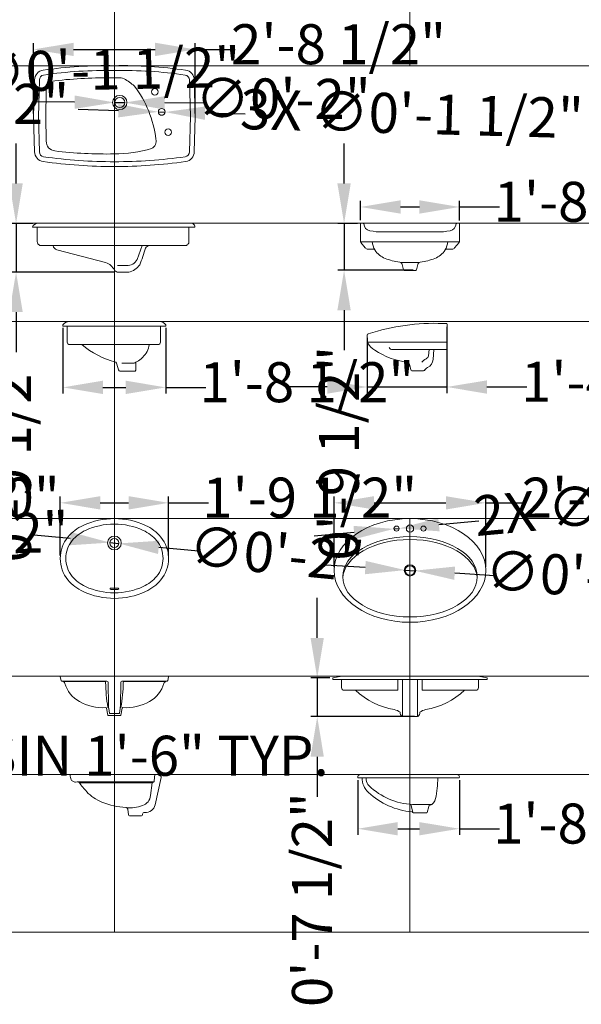
# Model space of a CAD drawing. Units: inches. Extents: x 2138 to 3265, y 2149 to 3392.
# Tile 8 of 13: x 2928 to 3040, y 3051 to 3248. Entities that reach past the tile are written whole.
import ezdxf

# ---------------------------------------------------------------- set-up
doc = ezdxf.new("R2010")
doc.units = ezdxf.units.IN
for name, color, linetype, lineweight in [('A-ANNO-DIMS', 2, 'Continuous', 18), ('A-DETL-GRID', 1, 'Continuous', 13), ('Washbasin-detail', 251, 'Continuous', 13), ('Washbasin-outline', 250, 'Continuous', 20)]:
    doc.layers.add(name, color=color, linetype=linetype, lineweight=lineweight)
doc.styles.get("Standard").update_dxf_attribs({"font": 'arial.ttf'})
doc.dimstyles.new('ISO-25', dxfattribs={"dimtxt": 8, "dimasz": 8, "dimexe": 1.25, "dimexo": 0.625, "dimtad": 0, "dimdec": 1, "dimlunit": 4, "dimtxsty": 'Standard', "dimcen": 2.5, "dimadec": 0, "dimazin": 0, "dimtfac": 1, "dimtdec": 1, "dimtmove": 0, "dimatfit": 3, "dimfxl": 1, "dimarcsym": 0})

# ---------------------------------------------------------------- blocks, each defined once
blk = doc.blocks.new('BASIN-WALLHUNG-SIDE')
for p, q in [((16.94, 8.23), (16.8, 6.96)), ((0.38, 6.97), (0.83, 6.75)), ((1.41, 6.77), (1.08, 6.71)), ((1.41, 6.77), (16.72, 6.77)), ((1.8, 6.61), (16.41, 6.61)), ((16.36, 6.61), (16.07, 4.02)), ((11.67, 0.17), (11.54, 1.3)), ((14.45, 0.17), (14.46, 0.29)), ((11.87, 0), (14.25, 0))]:
    blk.add_line(p, q)
for points in [[(17.61, 8.23), (0.08, 8.23, 0.427055), (0, 8.15, 0.060898), (0.18, 7.2)], [(17.81, 8.05), (18.01, 7.98, -0.38584), (18.2, 7.66), (16.99, 2.18)]]:
    blk.add_lwpolyline(points, format="xyb")
for centre, radius, start, end in [((17.61, 8.11), 0.119, 11.3189, 90), ((17.85, 8.16), 0.119, 191.3189, 251.9239), ((0.56, 7.33), 0.396, 197.6362, 243.4349), ((1.01, 7.1), 0.396, 243.4349, 279.8522), ((1.48, 6.38), 0.396, 36.3193, 99.8522), ((18.06, 18.57), 20.18, 216.3193, 223.028), ((16.41, 7.01), 0.396, 270, 353.6234), ((9.38, 10.47), 8.31, 223.028, 248.5761), ((13.71, 4.28), 2.37, 288.7646, 353.6234), ((12.27, 17.83), 16.23, 248.5761, 266.122), ((12.12, 7.8), 6.22, 261.2493, 292.2117), ((15.05, 2.61), 1.98, 265.1357, 347.5295), ((11.15, 1.25), 0.396, 6.7098, 86.122), ((11.87, 0.2), 0.198, 186.7098, 270), ((14.25, 0.2), 0.198, 270, 353.2902), ((14.85, 0.25), 0.396, 85.1357, 173.2902)]:
    blk.add_arc(centre, radius, start, end)
blk = doc.blocks.new('*D49')
at = {"layer": 'A-ANNO-DIMS', "color": 0, "lineweight": -2, "transparency": 16777216}
for p, q in [((2878.67, 3097.91), (2878.67, 3101.27)), ((2896.9, 3097.91), (2896.9, 3101.27)), ((2886.67, 3100.02), (2888.9, 3100.02)), ((2896.9, 3100.02), (2904.9, 3100.02))]:
    blk.add_line(p, q, dxfattribs=at)
at = {"layer": 'A-ANNO-DIMS', "color": 0, "transparency": 16777216}
for points in [[(2886.67, 3101.35), (2886.67, 3098.69), (2878.67, 3100.02)], [(2888.9, 3101.35), (2888.9, 3098.69), (2896.9, 3100.02)]]:
    blk.add_solid(points, dxfattribs=at)
at = {"layer": 'Defpoints', "color": 0, "transparency": 16777216}
for p in [(2896.9, 3100.02), (2878.67, 3097.29), (2896.9, 3097.29)]:
    blk.add_point(p, dxfattribs=at)
at = {"layer": 'A-ANNO-DIMS', "color": 0, "transparency": 16777216, "insert": (2948.05, 3100.02), "char_height": 8, "attachment_point": 5}
blk.add_mtext('BASIN 1\'-6" TYP.', dxfattribs=at)
blk = doc.blocks.new('*D82')
at = {"layer": 'A-ANNO-DIMS', "color": 0, "lineweight": -2, "transparency": 16777216}
for p, q in [((2930.43, 3229.45), (2930.43, 3243.52)), ((2938.43, 3242.27), (2954.71, 3242.27)), ((2962.71, 3229.45), (2962.71, 3243.52)), ((2962.71, 3242.27), (2970.71, 3242.27))]:
    blk.add_line(p, q, dxfattribs=at)
at = {"layer": 'A-ANNO-DIMS', "color": 0, "transparency": 16777216}
for points in [[(2938.43, 3243.6), (2938.43, 3240.94), (2930.43, 3242.27)], [(2954.71, 3243.6), (2954.71, 3240.94), (2962.71, 3242.27)]]:
    blk.add_solid(points, dxfattribs=at)
at = {"layer": 'Defpoints', "color": 0, "transparency": 16777216}
for p in [(2962.71, 3242.27), (2930.43, 3228.82), (2962.71, 3228.82)]:
    blk.add_point(p, dxfattribs=at)
at = {"layer": 'A-ANNO-DIMS', "color": 0, "transparency": 16777216, "insert": (2991.36, 3242.27), "char_height": 8, "attachment_point": 5}
blk.add_mtext('2\'-8 1/2"', dxfattribs=at)
blk = doc.blocks.new('*D83')
at = {"layer": 'A-ANNO-DIMS', "color": 0, "lineweight": -2, "transparency": 16777216}
for p, q in [((2926.93, 3215.47), (2926.93, 3223.47)), ((2930.28, 3207.47), (2925.68, 3207.47)), ((2926.93, 3207.47), (2926.93, 3197.76)), ((2946.5, 3197.76), (2925.68, 3197.76)), ((2926.93, 3189.76), (2926.93, 3181.76))]:
    blk.add_line(p, q, dxfattribs=at)
at = {"layer": 'A-ANNO-DIMS', "color": 0, "transparency": 16777216}
for points in [[(2925.59, 3215.47), (2928.26, 3215.47), (2926.93, 3207.47)], [(2925.59, 3189.76), (2928.26, 3189.76), (2926.93, 3197.76)]]:
    blk.add_solid(points, dxfattribs=at)
at = {"layer": 'Defpoints', "color": 0, "transparency": 16777216}
for p in [(2930.91, 3207.47), (2926.93, 3197.76), (2947.13, 3197.76)]:
    blk.add_point(p, dxfattribs=at)
at = {"layer": 'A-ANNO-DIMS', "color": 0, "transparency": 16777216, "insert": (2926.93, 3161.18), "char_height": 8, "attachment_point": 5, "rotation": 90}
blk.add_mtext('0\'-9 1/2"', dxfattribs=at)
blk = doc.blocks.new('*D84')
at = {"layer": 'A-ANNO-DIMS', "color": 0, "lineweight": -2, "transparency": 16777216}
for p, q in [((2936.28, 3186.58), (2936.28, 3173.45)), ((2956.83, 3186.58), (2956.83, 3173.45)), ((2944.28, 3174.7), (2948.83, 3174.7)), ((2956.83, 3174.7), (2964.83, 3174.7))]:
    blk.add_line(p, q, dxfattribs=at)
at = {"layer": 'A-ANNO-DIMS', "color": 0, "transparency": 16777216}
for points in [[(2944.28, 3176.04), (2944.28, 3173.37), (2936.28, 3174.7)], [(2948.83, 3176.04), (2948.83, 3173.37), (2956.83, 3174.7)]]:
    blk.add_solid(points, dxfattribs=at)
at = {"layer": 'Defpoints', "color": 0, "transparency": 16777216}
for p in [(2936.28, 3187.21), (2956.83, 3187.21), (2956.83, 3174.7)]:
    blk.add_point(p, dxfattribs=at)
at = {"layer": 'A-ANNO-DIMS', "color": 0, "transparency": 16777216, "insert": (2985.03, 3174.7), "char_height": 8, "attachment_point": 5}
blk.add_mtext('1\'-8 1/2"', dxfattribs=at)
blk = doc.blocks.new('*D85')
at = {"layer": 'A-ANNO-DIMS', "color": 0, "lineweight": -2, "transparency": 16777216}
for p, q in [((2995.75, 3208.1), (2995.75, 3212.02)), ((3003.75, 3210.77), (3007.52, 3210.77)), ((3015.52, 3208.08), (3015.52, 3212.02)), ((3015.52, 3210.77), (3023.52, 3210.77))]:
    blk.add_line(p, q, dxfattribs=at)
at = {"layer": 'A-ANNO-DIMS', "color": 0, "transparency": 16777216}
for points in [[(3003.75, 3212.11), (3003.75, 3209.44), (2995.75, 3210.77)], [(3007.52, 3212.11), (3007.52, 3209.44), (3015.52, 3210.77)]]:
    blk.add_solid(points, dxfattribs=at)
at = {"layer": 'Defpoints', "color": 0, "transparency": 16777216}
for p in [(3015.52, 3210.77), (2995.75, 3207.48), (3015.52, 3207.45)]:
    blk.add_point(p, dxfattribs=at)
at = {"layer": 'A-ANNO-DIMS', "color": 0, "transparency": 16777216, "insert": (3034.4, 3210.77), "char_height": 8, "attachment_point": 5}
blk.add_mtext('1\'-8"', dxfattribs=at)
blk = doc.blocks.new('*D86')
at = {"layer": 'A-ANNO-DIMS', "color": 0, "lineweight": -2, "transparency": 16777216}
for p, q in [((2992.46, 3215.48), (2992.46, 3223.48)), ((2995.13, 3207.48), (2991.21, 3207.48)), ((2992.46, 3207.48), (2992.46, 3198.12)), ((3006.25, 3198.12), (2991.21, 3198.12)), ((2992.46, 3190.12), (2992.46, 3182.12))]:
    blk.add_line(p, q, dxfattribs=at)
at = {"layer": 'A-ANNO-DIMS', "color": 0, "transparency": 16777216}
for points in [[(2991.12, 3215.48), (2993.79, 3215.48), (2992.46, 3207.48)], [(2991.12, 3190.12), (2993.79, 3190.12), (2992.46, 3198.12)]]:
    blk.add_solid(points, dxfattribs=at)
at = {"layer": 'Defpoints', "color": 0, "transparency": 16777216}
for p in [(2995.75, 3207.48), (2992.46, 3198.12), (3006.88, 3198.12)]:
    blk.add_point(p, dxfattribs=at)
at = {"layer": 'A-ANNO-DIMS', "color": 0, "transparency": 16777216, "insert": (2992.46, 3161.54), "char_height": 8, "attachment_point": 5, "rotation": 90}
blk.add_mtext('0\'-9 1/2"', dxfattribs=at)
blk = doc.blocks.new('*D87')
at = {"layer": 'A-ANNO-DIMS', "color": 0, "lineweight": -2, "transparency": 16777216}
for p, q in [((3012.99, 3186.82), (3012.99, 3173.53)), ((2997.1, 3184.61), (2997.1, 3173.53)), ((2989.1, 3174.78), (2981.1, 3174.78)), ((2997.1, 3174.78), (3012.99, 3174.78)), ((3020.99, 3174.78), (3028.99, 3174.78))]:
    blk.add_line(p, q, dxfattribs=at)
at = {"layer": 'A-ANNO-DIMS', "color": 0, "transparency": 16777216}
for points in [[(2989.1, 3176.11), (2989.1, 3173.44), (2997.1, 3174.78)], [(3020.99, 3176.11), (3020.99, 3173.44), (3012.99, 3174.78)]]:
    blk.add_solid(points, dxfattribs=at)
at = {"layer": 'Defpoints', "color": 0, "transparency": 16777216}
for p in [(3012.99, 3187.44), (2997.1, 3185.23), (3012.99, 3174.78)]:
    blk.add_point(p, dxfattribs=at)
at = {"layer": 'A-ANNO-DIMS', "color": 0, "transparency": 16777216, "insert": (3039.87, 3174.78), "char_height": 8, "attachment_point": 5}
blk.add_mtext('1\'-4"', dxfattribs=at)
blk = doc.blocks.new('*D89')
at = {"layer": 'A-ANNO-DIMS', "color": 0, "lineweight": -2, "transparency": 16777216}
for p, q in [((3048.17, 3215.38), (3048.17, 3223.38)), ((3050.93, 3207.38), (3046.92, 3207.38)), ((3048.17, 3207.38), (3048.17, 3199.85)), ((3065.38, 3199.85), (3046.92, 3199.85)), ((3048.17, 3191.85), (3048.17, 3183.85))]:
    blk.add_line(p, q, dxfattribs=at)
at = {"layer": 'A-ANNO-DIMS', "color": 0, "transparency": 16777216}
for points in [[(3046.84, 3215.38), (3049.5, 3215.38), (3048.17, 3207.38)], [(3046.84, 3191.85), (3049.5, 3191.85), (3048.17, 3199.85)]]:
    blk.add_solid(points, dxfattribs=at)
at = {"layer": 'Defpoints', "color": 0, "transparency": 16777216}
for p in [(3051.56, 3207.38), (3048.17, 3199.85), (3066, 3199.85)]:
    blk.add_point(p, dxfattribs=at)
at = {"layer": 'A-ANNO-DIMS', "color": 0, "transparency": 16777216, "insert": (3048.17, 3163.27), "char_height": 8, "attachment_point": 5, "rotation": 90}
blk.add_mtext('0\'-7 1/2"', dxfattribs=at)
blk = doc.blocks.new('*D97')
at = {"layer": 'A-ANNO-DIMS', "color": 0, "lineweight": -2, "transparency": 16777216}
for p, q in [((2876.44, 3139.39), (2876.44, 3152.87)), ((2898.59, 3139.39), (2898.59, 3152.87)), ((2884.44, 3151.62), (2890.59, 3151.62)), ((2898.59, 3151.62), (2906.59, 3151.62))]:
    blk.add_line(p, q, dxfattribs=at)
at = {"layer": 'A-ANNO-DIMS', "color": 0, "transparency": 16777216}
for points in [[(2884.44, 3152.95), (2884.44, 3150.28), (2876.44, 3151.62)], [(2890.59, 3152.95), (2890.59, 3150.28), (2898.59, 3151.62)]]:
    blk.add_solid(points, dxfattribs=at)
at = {"layer": 'Defpoints', "color": 0, "transparency": 16777216}
for p in [(2898.59, 3151.62), (2876.44, 3138.77), (2898.59, 3138.77)]:
    blk.add_point(p, dxfattribs=at)
at = {"layer": 'A-ANNO-DIMS', "color": 0, "transparency": 16777216, "insert": (2920.58, 3151.62), "char_height": 8, "attachment_point": 5}
blk.add_mtext('1\'-10"', dxfattribs=at)
blk = doc.blocks.new('*D98')
at = {"layer": 'A-ANNO-DIMS', "color": 0, "lineweight": -2, "transparency": 16777216}
for p, q in [((2935.75, 3141.12), (2935.75, 3152.87)), ((2957.4, 3141.12), (2957.4, 3152.87)), ((2943.75, 3151.62), (2949.4, 3151.62)), ((2957.4, 3151.62), (2965.4, 3151.62))]:
    blk.add_line(p, q, dxfattribs=at)
at = {"layer": 'A-ANNO-DIMS', "color": 0, "transparency": 16777216}
for points in [[(2943.75, 3152.95), (2943.75, 3150.28), (2935.75, 3151.62)], [(2949.4, 3152.95), (2949.4, 3150.28), (2957.4, 3151.62)]]:
    blk.add_solid(points, dxfattribs=at)
at = {"layer": 'Defpoints', "color": 0, "transparency": 16777216}
for p in [(2957.4, 3151.62), (2935.75, 3140.5), (2957.4, 3140.5)]:
    blk.add_point(p, dxfattribs=at)
at = {"layer": 'A-ANNO-DIMS', "color": 0, "transparency": 16777216, "insert": (2985.6, 3151.62), "char_height": 8, "attachment_point": 5}
blk.add_mtext('1\'-9 1/2"', dxfattribs=at)
blk = doc.blocks.new('*D99')
at = {"layer": 'A-ANNO-DIMS', "color": 0, "lineweight": -2, "transparency": 16777216}
for p, q in [((2990.46, 3138.73), (2990.46, 3152.87)), ((3020.79, 3138.73), (3020.79, 3152.87)), ((2998.46, 3151.62), (3012.79, 3151.62)), ((3020.79, 3151.62), (3028.79, 3151.62))]:
    blk.add_line(p, q, dxfattribs=at)
at = {"layer": 'A-ANNO-DIMS', "color": 0, "transparency": 16777216}
for points in [[(2998.46, 3152.95), (2998.46, 3150.28), (2990.46, 3151.62)], [(3012.79, 3152.95), (3012.79, 3150.28), (3020.79, 3151.62)]]:
    blk.add_solid(points, dxfattribs=at)
at = {"layer": 'Defpoints', "color": 0, "transparency": 16777216}
for p in [(3020.79, 3151.62), (2990.46, 3138.1), (3020.79, 3138.1)]:
    blk.add_point(p, dxfattribs=at)
at = {"layer": 'A-ANNO-DIMS', "color": 0, "transparency": 16777216, "insert": (3049.44, 3151.62), "char_height": 8, "attachment_point": 5}
blk.add_mtext('2\'-6 1/2"', dxfattribs=at)
blk = doc.blocks.new('*D100')
at = {"layer": 'A-ANNO-DIMS', "color": 0, "lineweight": -2, "transparency": 16777216}
for p, q in [((2987.09, 3124.6), (2987.09, 3132.6)), ((2989.61, 3116.6), (2985.84, 3116.6)), ((2987.09, 3116.6), (2987.09, 3108.87)), ((3006.53, 3108.87), (2985.84, 3108.87)), ((2987.09, 3100.87), (2987.09, 3092.87))]:
    blk.add_line(p, q, dxfattribs=at)
at = {"layer": 'A-ANNO-DIMS', "color": 0, "transparency": 16777216}
for points in [[(2985.76, 3124.6), (2988.42, 3124.6), (2987.09, 3116.6)], [(2985.76, 3100.87), (2988.42, 3100.87), (2987.09, 3108.87)]]:
    blk.add_solid(points, dxfattribs=at)
at = {"layer": 'Defpoints', "color": 0, "transparency": 16777216}
for p in [(2990.24, 3116.6), (2987.09, 3108.87), (3007.15, 3108.87)]:
    blk.add_point(p, dxfattribs=at)
at = {"layer": 'A-ANNO-DIMS', "color": 0, "transparency": 16777216, "insert": (2987.09, 3072.29), "char_height": 8, "attachment_point": 5, "rotation": 90}
blk.add_mtext('0\'-7 1/2"', dxfattribs=at)
blk = doc.blocks.new('*D101')
at = {"layer": 'A-ANNO-DIMS', "color": 0, "lineweight": -2, "transparency": 16777216}
for p, q in [((2995.19, 3096.14), (2995.19, 3085.21)), ((3015.5, 3096.19), (3015.5, 3085.21)), ((3003.19, 3086.46), (3007.5, 3086.46)), ((3015.5, 3086.46), (3023.5, 3086.46))]:
    blk.add_line(p, q, dxfattribs=at)
at = {"layer": 'A-ANNO-DIMS', "color": 0, "transparency": 16777216}
for points in [[(3003.19, 3087.79), (3003.19, 3085.13), (2995.19, 3086.46)], [(3007.5, 3087.79), (3007.5, 3085.13), (3015.5, 3086.46)]]:
    blk.add_solid(points, dxfattribs=at)
at = {"layer": 'Defpoints', "color": 0, "transparency": 16777216}
for p in [(2995.19, 3096.77), (3015.5, 3096.81), (3015.5, 3086.46)]:
    blk.add_point(p, dxfattribs=at)
at = {"layer": 'A-ANNO-DIMS', "color": 0, "transparency": 16777216, "insert": (3043.7, 3086.46), "char_height": 8, "attachment_point": 5}
blk.add_mtext('1\'-8 1/2"', dxfattribs=at)
blk = doc.blocks.new('*D121')
at = {"layer": 'A-ANNO-DIMS', "color": 0, "lineweight": -2, "transparency": 16777216}
for p, q in [((2904.18, 3236.4), (2896.19, 3236.24)), ((2878.85, 3235.89), (2870.85, 3235.74)), ((2886.85, 3236.05), (2888.19, 3236.08))]:
    blk.add_line(p, q, dxfattribs=at)
at = {"layer": 'A-ANNO-DIMS', "color": 0, "transparency": 16777216}
for points in [[(2878.82, 3237.23), (2878.88, 3234.56), (2886.85, 3236.05)], [(2896.16, 3237.57), (2896.21, 3234.91), (2888.19, 3236.08)]]:
    blk.add_solid(points, dxfattribs=at)
at = {"layer": 'Defpoints', "color": 0, "transparency": 16777216}
for p in [(2886.85, 3236.05), (2888.19, 3236.08)]:
    blk.add_point(p, dxfattribs=at)
at = {"layer": 'A-ANNO-DIMS', "color": 0, "transparency": 16777216, "insert": (2937.49, 3237.06), "char_height": 8, "attachment_point": 5, "rotation": 1.1379}
blk.add_mtext('3X ∅0\'-1 1/2"', dxfattribs=at)
blk = doc.blocks.new('*D122')
at = {"layer": 'A-ANNO-DIMS', "color": 0, "lineweight": -2, "transparency": 16777216}
for p, q in [((2878.63, 3230.6), (2870.63, 3230.64)), ((2886.63, 3230.56), (2888.4, 3230.55)), ((2904.4, 3230.47), (2896.4, 3230.51))]:
    blk.add_line(p, q, dxfattribs=at)
at = {"layer": 'A-ANNO-DIMS', "color": 0, "transparency": 16777216}
for points in [[(2878.64, 3231.93), (2878.63, 3229.27), (2886.63, 3230.56)], [(2896.41, 3231.84), (2896.4, 3229.18), (2888.4, 3230.55)]]:
    blk.add_solid(points, dxfattribs=at)
at = {"layer": 'Defpoints', "color": 0, "transparency": 16777216}
for p in [(2886.63, 3230.56), (2888.4, 3230.55)]:
    blk.add_point(p, dxfattribs=at)
at = {"layer": 'A-ANNO-DIMS', "color": 0, "transparency": 16777216, "insert": (2920.01, 3230.39), "char_height": 8, "attachment_point": 5, "rotation": 359.7153}
blk.add_mtext('∅0\'-2"', dxfattribs=at)
blk = doc.blocks.new('*D123')
at = {"layer": 'A-ANNO-DIMS', "color": 0, "lineweight": -2, "transparency": 16777216}
for p, q in [((2947.36, 3230.01), (2939.36, 3230.23)), ((2955.35, 3229.79), (2956.69, 3229.75)), ((2972.68, 3229.31), (2964.69, 3229.53))]:
    blk.add_line(p, q, dxfattribs=at)
at = {"layer": 'A-ANNO-DIMS', "color": 0, "transparency": 16777216}
for points in [[(2947.39, 3231.34), (2947.32, 3228.67), (2955.35, 3229.79)], [(2964.72, 3230.86), (2964.65, 3228.19), (2956.69, 3229.75)]]:
    blk.add_solid(points, dxfattribs=at)
at = {"layer": 'Defpoints', "color": 0, "transparency": 16777216}
for p in [(2955.35, 3229.79), (2956.69, 3229.75)]:
    blk.add_point(p, dxfattribs=at)
at = {"layer": 'A-ANNO-DIMS', "color": 0, "transparency": 16777216, "insert": (3005.98, 3228.39), "char_height": 8, "attachment_point": 5, "rotation": 358.4162}
blk.add_mtext('3X ∅0\'-1 1/2"', dxfattribs=at)
blk = doc.blocks.new('*D124')
at = {"layer": 'A-ANNO-DIMS', "color": 0, "lineweight": -2, "transparency": 16777216}
for p, q in [((2938.63, 3231.73), (2930.63, 3231.79)), ((2946.63, 3231.66), (2948.64, 3231.65)), ((2964.64, 3231.52), (2956.64, 3231.59))]:
    blk.add_line(p, q, dxfattribs=at)
at = {"layer": 'A-ANNO-DIMS', "color": 0, "transparency": 16777216}
for points in [[(2938.64, 3233.06), (2938.62, 3230.39), (2946.63, 3231.66)], [(2956.65, 3232.92), (2956.63, 3230.25), (2948.64, 3231.65)]]:
    blk.add_solid(points, dxfattribs=at)
at = {"layer": 'Defpoints', "color": 0, "transparency": 16777216}
for p in [(2946.63, 3231.66), (2948.64, 3231.65)]:
    blk.add_point(p, dxfattribs=at)
at = {"layer": 'A-ANNO-DIMS', "color": 0, "transparency": 16777216, "insert": (2980.25, 3231.4), "char_height": 8, "attachment_point": 5, "rotation": 359.5528}
blk.add_mtext('∅0\'-2"', dxfattribs=at)
blk = doc.blocks.new('*D130')
at = {"layer": 'A-ANNO-DIMS', "color": 0, "lineweight": -2, "transparency": 16777216}
for p, q in [((2904.4, 3143.83), (2896.4, 3143.59)), ((2878.63, 3143.06), (2870.63, 3142.82)), ((2886.63, 3143.3), (2888.41, 3143.35))]:
    blk.add_line(p, q, dxfattribs=at)
at = {"layer": 'A-ANNO-DIMS', "color": 0, "transparency": 16777216}
for points in [[(2878.59, 3144.39), (2878.67, 3141.72), (2886.63, 3143.3)], [(2896.36, 3144.92), (2896.44, 3142.26), (2888.41, 3143.35)]]:
    blk.add_solid(points, dxfattribs=at)
at = {"layer": 'Defpoints', "color": 0, "transparency": 16777216}
for p in [(2886.63, 3143.3), (2888.41, 3143.35)]:
    blk.add_point(p, dxfattribs=at)
at = {"layer": 'A-ANNO-DIMS', "color": 0, "transparency": 16777216, "insert": (2920, 3144.3), "char_height": 8, "attachment_point": 5, "rotation": 1.7228}
blk.add_mtext('∅0\'-2"', dxfattribs=at)
blk = doc.blocks.new('*D131')
at = {"layer": 'A-ANNO-DIMS', "color": 0, "lineweight": -2, "transparency": 16777216}
for p, q in [((2937.73, 3144.46), (2929.77, 3145.24)), ((2945.69, 3143.67), (2947.45, 3143.5)), ((2963.38, 3141.93), (2955.42, 3142.72))]:
    blk.add_line(p, q, dxfattribs=at)
at = {"layer": 'A-ANNO-DIMS', "color": 0, "transparency": 16777216}
for points in [[(2937.86, 3145.78), (2937.6, 3143.13), (2945.69, 3143.67)], [(2955.55, 3144.04), (2955.29, 3141.39), (2947.45, 3143.5)]]:
    blk.add_solid(points, dxfattribs=at)
at = {"layer": 'Defpoints', "color": 0, "transparency": 16777216}
for p in [(2945.69, 3143.67), (2947.45, 3143.5)]:
    blk.add_point(p, dxfattribs=at)
at = {"layer": 'A-ANNO-DIMS', "color": 0, "transparency": 16777216, "insert": (2978.91, 3140.41), "char_height": 8, "attachment_point": 5, "rotation": 354.3826}
blk.add_mtext('∅0\'-2"', dxfattribs=at)
blk = doc.blocks.new('*D132')
at = {"layer": 'A-ANNO-DIMS', "color": 0, "lineweight": -2, "transparency": 16777216}
for p, q in [((3019.38, 3147.98), (3011.42, 3147.24)), ((3002.43, 3146.42), (3003.45, 3146.51)), ((2994.46, 3145.69), (2986.49, 3144.95))]:
    blk.add_line(p, q, dxfattribs=at)
at = {"layer": 'A-ANNO-DIMS', "color": 0, "transparency": 16777216}
for points in [[(3011.29, 3148.57), (3011.54, 3145.92), (3003.45, 3146.51)], [(2994.34, 3147.01), (2994.58, 3144.36), (3002.43, 3146.42)]]:
    blk.add_solid(points, dxfattribs=at)
at = {"layer": 'Defpoints', "color": 0, "transparency": 16777216}
for p in [(3002.43, 3146.42), (3003.45, 3146.51)]:
    blk.add_point(p, dxfattribs=at)
at = {"layer": 'A-ANNO-DIMS', "color": 0, "transparency": 16777216, "insert": (3043.34, 3150.18), "char_height": 8, "attachment_point": 5, "rotation": 5.2513}
blk.add_mtext('2X ∅0\'-1"', dxfattribs=at)
blk = doc.blocks.new('*D133')
at = {"layer": 'A-ANNO-DIMS', "color": 0, "lineweight": -2, "transparency": 16777216}
for p, q in [((2996.7, 3138.67), (2988.72, 3139.17)), ((3004.68, 3138.17), (3006.57, 3138.05)), ((3022.54, 3137.05), (3014.56, 3137.55))]:
    blk.add_line(p, q, dxfattribs=at)
at = {"layer": 'A-ANNO-DIMS', "color": 0, "transparency": 16777216}
for points in [[(2996.78, 3140), (2996.62, 3137.34), (3004.68, 3138.17)], [(3014.64, 3138.88), (3014.47, 3136.22), (3006.57, 3138.05)]]:
    blk.add_solid(points, dxfattribs=at)
at = {"layer": 'Defpoints', "color": 0, "transparency": 16777216}
for p in [(3004.68, 3138.17), (3006.57, 3138.05)]:
    blk.add_point(p, dxfattribs=at)
at = {"layer": 'A-ANNO-DIMS', "color": 0, "transparency": 16777216, "insert": (3038.12, 3136.08), "char_height": 8, "attachment_point": 5, "rotation": 356.4158}
blk.add_mtext('∅0\'-2"', dxfattribs=at)

msp = doc.modelspace()

# ---------------------------------------------------------------- linework, layer by layer
at = {"layer": 'A-DETL-GRID'}
for p, q in [((2946.57, 3239.02), (2946.57, 3370.91)), ((3005.63, 3239.02), (3005.63, 3370.91)), ((2828.46, 3239.02), (3241.85, 3239.02)), ((2828.46, 3239.02), (3241.85, 3239.02)), ((2946.57, 3148.47), (2946.57, 3239.02)), ((2828.46, 3207.52), (3241.85, 3207.52)), ((2828.46, 3187.84), (3241.85, 3187.84)), ((2828.46, 3148.47), (3241.85, 3148.47)), ((2828.46, 3148.47), (3241.85, 3148.47)), ((2946.57, 3065.79), (2946.57, 3148.47)), ((3005.63, 3065.79), (3005.63, 3148.47)), ((2828.46, 3116.97), (3241.85, 3116.97)), ((2828.46, 3097.29), (3241.85, 3097.29)), ((2828.46, 3065.79), (3241.85, 3065.79))]:
    msp.add_line(p, q, dxfattribs=at)
at = {"layer": 'Washbasin-detail'}
for p, q in [((2961.75, 3228.8), (2961.55, 3236.16)), ((2931.4, 3228.85), (2931.6, 3221.8)), ((2961.75, 3228.85), (2961.55, 3221.8)), ((2996.26, 3207.52), (3005.63, 3207.52)), ((3005.63, 3207.52), (3015, 3207.52)), ((2997.11, 3183.76), (3013.03, 3183.76)), ((3009.44, 3182.28), (3009.31, 3181.04)), ((3008.4, 3180.11), (3008.01, 3179.72)), ((2946.57, 3134.59), (2945.85, 3134.59)), ((2946.57, 3134.29), (2945.85, 3134.29)), ((2946.57, 3134.59), (2947.29, 3134.59)), ((2946.57, 3134.29), (2947.29, 3134.29)), ((2936.45, 3115.87), (2944.66, 3115.87)), ((2936.51, 3115.87), (2944.66, 3115.87)), ((2956.64, 3115.87), (2948.48, 3115.87)), ((2956.7, 3115.87), (2948.49, 3115.87))]:
    msp.add_line(p, q, dxfattribs=at)
for points in [[(2946.55, 3238.05, 0.041442), (2932.43, 3237.15, 0.364581), (2931.6, 3236.16), (2931.4, 3228.8)], [(2946.59, 3238.05, -0.041442), (2960.72, 3237.15, -0.364581), (2961.55, 3236.16, -0.365525)], [(2946.59, 3219.82, -0.035481), (2932.43, 3220.81, -0.364581), (2931.6, 3221.8, -0.365525)], [(2946.59, 3219.82, 0.035408), (2960.72, 3220.81, 0.364581), (2961.55, 3221.8, 0.365525)], [(2934.31, 3203.04, 0.219637), (2935.1, 3202.17), (2944.82, 3199.65, -0.213245), (2946.59, 3198.11, 0.195887), (2947.34, 3197.72), (2949.43, 3197.72, 0.173732), (2951.63, 3199.18, 0.026954), (2952.77, 3202.56, -0.212214), (2953.56, 3203.04, -2.257631)], [(2952.1, 3203.04), (2951.12, 3200.28, -0.284687), (2948.99, 3199.06), (2947.22, 3199.06)], [(2940.06, 3183.27, 0.112903), (2946.87, 3179.73, -0.192582), (2947.07, 3179.37), (2947.42, 3178.19, 0.369924), (2947.66, 3177.96), (2948.08, 3177.96, 0.463799)], [(2952.23, 3180.71, 0.150901), (2953.56, 3183.27, -11.163636)], [(2948.05, 3179.57), (2950.49, 3179.57, 0.019838), (2950.85, 3179.72, -11.163636)], [(2950.15, 3177.96), (2950.61, 3177.96, 0.463799), (2950.84, 3178.15), (2950.84, 3179.73)], [(2950.85, 3179.72, 0.064766), (2951.91, 3180.41, -11.163636)], [(2951.91, 3180.41, 0.022705), (2952.23, 3180.71, -11.163636)], [(2948.08, 3177.96), (2950.15, 3177.96, 0.463799)], [(2991.94, 3116.31), (2991.94, 3114.71, 0.414442), (2992.5, 3114.14), (2994.73, 3114.14)], [(3019.32, 3116.31), (3019.32, 3114.71, -0.414442), (3018.75, 3114.14), (3016.53, 3114.14)], [(3004.06, 3108.91, -0.32061), (3003.68, 3109.76, 0.099522), (3002.5, 3110.28, -0.147273), (2994.73, 3114.14, -6.747866)], [(3007.2, 3108.91, 0.32061), (3007.58, 3109.76, -0.099522), (3008.75, 3110.28, 0.147273), (3016.53, 3114.14, 6.747866)]]:
    msp.add_lwpolyline(points, format="xyb", dxfattribs=at)
for points in [[(2994.73, 3114.14), (3003.21, 3114.14), (3003.21, 3116.31)], [(3004.11, 3116.31), (3004.11, 3108.91)], [(3007.15, 3116.31), (3007.15, 3108.87)], [(3016.53, 3114.14), (3008.05, 3114.14), (3008.05, 3116.31)], [(3004.11, 3108.91), (3004.11, 3108.87), (3005.63, 3108.87)], [(3007.15, 3108.87), (3005.63, 3108.87)]]:
    msp.add_lwpolyline(points, dxfattribs=at)
for centre, radius in [((2954.64, 3233.8), 0.669), ((2947.64, 3231.66), 1.43), ((2947.64, 3231.66), 1), ((2956.02, 3229.77), 0.669), ((2957.32, 3225.73), 0.669), ((3002.94, 3146.47), 0.514), ((3005.63, 3146.47), 0.727), ((3008.32, 3146.47), 0.514), ((2946.57, 3143.59), 0.886), ((3005.63, 3138.11), 1.14), ((3005.63, 3138.11), 0.945)]:
    msp.add_circle(centre, radius, dxfattribs=at)
for centre, radius, start, end in [((3002.14, 3204.33), 4.12, 186.9142, 211.518), ((3009.12, 3204.33), 4.12, 328.482, 353.0858), ((3005.19, 3212.24), 12.6, 262.6134, 272.0037), ((3006.07, 3212.24), 12.6, 267.9963, 277.3866), ((3009.69, 3178.63), 1.97, 115.0744, 130.9196), ((3008.52, 3181.12), 0.787, 295.0744, 354.0175), ((2943.95, 3139.24), 7.56, 114.5967, 140.1807), ((2946.57, 3133.51), 13.86, 90, 114.5967), ((2946.57, 3133.51), 13.86, 65.4033, 90), ((2949.19, 3139.24), 7.56, 39.8193, 65.4033), ((2942.44, 3140.5), 5.59, 140.1807, 180), ((2946.57, 3143.59), 1.38, 90.0179, 269.9821), ((2946.57, 3143.59), 1.38, 270.0179, 89.9821), ((2950.71, 3140.5), 5.59, 0, 39.8193), ((2942.44, 3140.5), 5.59, 180, 219.8193), ((2950.71, 3140.5), 5.59, 320.1807, 0), ((2943.95, 3141.76), 7.56, 219.8193, 245.4033), ((2949.19, 3141.76), 7.56, 294.5967, 320.1807), ((2946.57, 3147.48), 13.86, 245.4033, 270), ((2945.85, 3134.44), 0.148, 90, 270), ((2946.57, 3147.48), 13.86, 270, 294.5967), ((2947.29, 3134.44), 0.148, 270, 90), ((2944.66, 3115.71), 0.157, 0.8583, 90), ((2976.31, 3116.19), 31.5, 180.8583, 189.9879), ((2916.84, 3116.19), 31.5, 350.0121, 359.1417), ((2948.49, 3115.71), 0.157, 90, 179.1417), ((2945.37, 3110.74), 0.0787, 189.9879, 245.8354), ((2945.27, 3110.52), 0.157, 9.3709, 65.8354), ((2947.88, 3110.52), 0.157, 114.1646, 170.6291), ((2947.78, 3110.74), 0.0787, 294.1646, 350.0121), ((2999.99, 3096.62), 3.94, 180, 227.2665), ((3007.47, 3104.71), 14.96, 227.2665, 264.5027)]:
    msp.add_arc(centre, radius, start, end, dxfattribs=at)
msp.add_ellipse((3005.63, 3136.25), major_axis=(-13.45, 0), ratio=0.596831, start_param=3.178385, end_param=6.246393, dxfattribs=at)
at = {"layer": 'Washbasin-outline'}
for p, q in [((2930.43, 3228.82), (2930.63, 3236.16)), ((2962.71, 3228.82), (2962.52, 3236.16)), ((2932.94, 3234.03), (2932.86, 3228.82)), ((2930.43, 3228.82), (2930.63, 3221.8)), ((2932.94, 3223.93), (2932.86, 3228.82)), ((2962.71, 3228.82), (2962.52, 3221.8)), ((2995.71, 3204.03), (2995.71, 3207.37)), ((2995.86, 3207.52), (2996.26, 3207.52)), ((3015, 3207.52), (3015.39, 3207.52)), ((3015.55, 3207.37), (3015.55, 3204.03)), ((3000.23, 3205.79), (3005.63, 3205.79)), ((3011.02, 3205.79), (3005.63, 3205.79)), ((2995.74, 3203.83), (3005.63, 3203.83)), ((2996.7, 3202.58), (2995.84, 3203.66)), ((3015.52, 3203.83), (3005.63, 3203.83)), ((3015.42, 3203.66), (3014.55, 3202.58)), ((2998.36, 3202.33), (2997.23, 3202.33)), ((3014.03, 3202.33), (3012.9, 3202.33)), ((3004.31, 3198.23), (3004.07, 3199.29)), ((3006.95, 3198.23), (3007.19, 3199.29)), ((3004.49, 3198.07), (3005.63, 3198.07)), ((3006.77, 3198.07), (3005.63, 3198.07)), ((3012.19, 3187.48), (3012.91, 3187.48)), ((3013.03, 3187.36), (3013.03, 3182.48)), ((2997.08, 3185.13), (2997.08, 3183.98)), ((3002.16, 3182.28), (3010.36, 3182.28)), ((3010.25, 3180.3), (3010.36, 3182.28)), ((3010.36, 3182.28), (3012.83, 3182.28)), ((3005.81, 3178.18), (3005.56, 3179.31)), ((3006, 3178.03), (3008.32, 3178.03)), ((2935.75, 3116.83), (2935.92, 3116.09)), ((2935.86, 3116.97), (2946.57, 3116.97)), ((2957.28, 3116.97), (2946.57, 3116.97)), ((2957.4, 3116.83), (2957.23, 3116.09)), ((2936, 3115.99), (2945.07, 3115.99)), ((2936.27, 3115.93), (2936.05, 3115.97)), ((2936.07, 3115.99), (2945.07, 3115.99)), ((2936.07, 3115.99), (2945.07, 3115.99)), ((2936.07, 3115.99), (2945.07, 3115.99)), ((2945.39, 3110.98), (2945.31, 3115.76)), ((2947.76, 3110.98), (2947.84, 3115.76)), ((2957.15, 3115.99), (2948.08, 3115.99)), ((2957.07, 3115.99), (2948.08, 3115.99)), ((2957.07, 3115.99), (2948.08, 3115.99)), ((2957.07, 3115.99), (2948.08, 3115.99)), ((2956.87, 3115.93), (2957.1, 3115.97)), ((2945.28, 3109.16), (2945.02, 3110.54)), ((2945.43, 3110.52), (2945.58, 3109.58)), ((2947.72, 3110.52), (2947.56, 3109.58)), ((2947.86, 3109.16), (2948.12, 3110.54)), ((2945.36, 3109.1), (2946.57, 3109.1)), ((2945.73, 3109.49), (2946.57, 3109.49)), ((2947.42, 3109.49), (2946.57, 3109.49)), ((2947.79, 3109.1), (2946.57, 3109.1)), ((2995.19, 3096.74), (2995.19, 3096.77)), ((2995.3, 3096.62), (3011.22, 3096.62)), ((2996.23, 3097.29), (3015.03, 3097.29)), ((3011.22, 3096.62), (3015.38, 3096.62)), ((3015.5, 3096.81), (3015.5, 3096.74)), ((3006.22, 3089.7), (3005.77, 3091.36)), ((3007.51, 3091.33), (3006.13, 3091.33)), ((3007.51, 3091.33), (3010.01, 3091.33)), ((3009.03, 3089.7), (3009.37, 3090.94)), ((3006.34, 3089.61), (3008.91, 3089.61))]:
    msp.add_line(p, q, dxfattribs=at)
for points in [[(2946.57, 3239.02, 0.041258), (2932.35, 3238.11, 0.377432), (2930.63, 3236.16)], [(2946.57, 3239.02, -0.041258), (2960.8, 3238.11, -0.377432), (2962.52, 3236.16)], [(2946.53, 3221.37, 0.071516), (2954.01, 3222.48, 0.35453), (2954.88, 3224.33, 0.132812), (2950.55, 3234.96, 0.040841), (2948.54, 3236.42, 0.110865), (2947.24, 3236.58), (2946.53, 3236.59)], [(2946.57, 3218.84, -0.034265), (2932.35, 3219.85, -0.377432), (2930.63, 3221.8)], [(2946.57, 3218.84, 0.034272), (2960.8, 3219.85, 0.377432), (2962.52, 3221.8)], [(2961.47, 3206.7), (2962.66, 3206.7, 0.437518), (2961.87, 3207.52), (2931.28, 3207.52, 0.343108), (2930.18, 3206.7, 1.30925)], [(2930.18, 3206.7), (2931.16, 3206.7, 0.437518)], [(2931.16, 3206.7), (2961.47, 3206.7, 0.437518)], [(2931.16, 3206.7), (2931.16, 3203.82, 0.414214), (2931.95, 3203.04), (2934.31, 3203.04, 0.414214)], [(2953.56, 3203.04), (2960.69, 3203.04, 0.414214), (2961.47, 3203.82), (2961.47, 3206.7)], [(2934.31, 3203.04), (2953.56, 3203.04, 0.414214)], [(2937.14, 3186.97), (2936.28, 3186.97), (2936.28, 3187.21, -0.253728), (2937.54, 3187.84), (2955.61, 3187.84, -0.218251), (2956.83, 3187.21), (2956.83, 3186.97)], [(2937.14, 3186.97), (2937.14, 3183.74, 0.414214), (2937.62, 3183.27), (2940.06, 3183.27, 0.414214)], [(2953.56, 3183.27), (2955.29, 3183.27, 0.414214), (2955.77, 3183.74), (2955.77, 3186.97)], [(2940.06, 3183.27), (2953.56, 3183.27, 0.414214)]]:
    msp.add_lwpolyline(points, format="xyb", dxfattribs=at)
for points in [[(2955.77, 3186.97), (2937.14, 3186.97)], [(2956.83, 3186.97), (2955.77, 3186.97)], [(3005.63, 3116.97), (2992.03, 3116.97), (2990.24, 3116.6)], [(2990.24, 3116.6), (2990.24, 3116.31), (2991.94, 3116.31)], [(2991.94, 3116.31), (3005.63, 3116.31)], [(3005.63, 3116.97), (3019.23, 3116.97), (3021.02, 3116.6)], [(3019.32, 3116.31), (3005.63, 3116.31)], [(3021.02, 3116.6), (3021.02, 3116.31), (3019.32, 3116.31)]]:
    msp.add_lwpolyline(points, dxfattribs=at)
for centre, radius, start, end in [((2945.06, 3147.96), 88.64, 89.0474, 96.723), ((2934.91, 3234.03), 1.97, 96.7008, 180), ((2934.91, 3223.93), 1.97, 180, 263.2992), ((2945.06, 3310), 88.64, 263.277, 270.9526), ((2995.86, 3207.37), 0.157, 90, 180), ((2996.26, 3207.37), 0.157, 2.8626, 90), ((2997.87, 3207.45), 1.46, 182.8626, 258.6995), ((3013.38, 3207.45), 1.46, 281.3005, 357.1374), ((3015, 3207.37), 0.157, 90, 177.1374), ((3015.39, 3207.37), 0.157, 0, 90), ((2999.9, 3217.6), 11.81, 258.6995, 271.6153), ((3011.35, 3217.6), 11.81, 268.3847, 281.3005), ((2996.3, 3204.03), 0.591, 180, 218.6598), ((3014.96, 3204.03), 0.591, 321.3402, 360), ((2997.23, 3203), 0.669, 218.6598, 270), ((2998.36, 3202.01), 0.315, 31.518, 90), ((3002.14, 3204.33), 4.12, 211.518, 249.0081), ((3009.12, 3204.33), 4.12, 290.9919, 328.482), ((3012.9, 3202.01), 0.315, 90, 148.482), ((3014.03, 3203), 0.669, 270, 321.3402), ((3005.19, 3212.24), 12.6, 248.8726, 262.6134), ((3003.49, 3199.16), 0.591, 12.8586, 82.6134), ((3007.76, 3199.16), 0.591, 97.3866, 167.1414), ((3006.07, 3212.24), 12.6, 277.3866, 291.1274), ((3004.5, 3198.27), 0.197, 192.8586, 270), ((3006.75, 3198.27), 0.197, 270, 347.1414), ((3010.58, 3144.2), 43.31, 87.8768, 107.8548), ((3012.91, 3187.36), 0.118, 0, 90), ((2997.38, 3185.13), 0.295, 104.0604, 180), ((2997.87, 3183.98), 0.787, 180, 212.0568), ((3001.21, 3186.07), 4.72, 212.0568, 236.6515), ((3006.83, 3194.62), 14.96, 236.6515, 263.1661), ((3002.11, 3183.03), 0.754, 209.6966, 273.846), ((3012.83, 3182.48), 0.197, 270, 0), ((3004.98, 3179.18), 0.591, 12.4449, 83.1661), ((3008.28, 3180.42), 1.97, 295.8335, 356.5733), ((3006, 3178.22), 0.197, 192.4449, 270), ((3008.36, 3178.22), 0.197, 270, 325.9607), ((3009.82, 3177.23), 1.57, 115.8335, 145.9607), ((2946.57, 3133.51), 14.96, 90, 114.5967), ((2946.57, 3133.51), 14.96, 65.4033, 90), ((2943.95, 3139.24), 8.66, 114.5967, 140.1807), ((2949.19, 3139.24), 8.66, 39.8193, 65.4033), ((2942.44, 3140.5), 6.69, 140.1807, 180), ((2950.71, 3140.5), 6.69, 0, 39.8193), ((2942.44, 3140.5), 6.69, 180, 219.8193), ((2950.71, 3140.5), 6.69, 320.1807, 0), ((2943.95, 3141.76), 8.66, 219.8193, 245.4033), ((2949.19, 3141.76), 8.66, 294.5967, 320.1807), ((2946.57, 3147.48), 14.96, 245.4033, 270), ((2946.57, 3147.48), 14.96, 270, 294.5967), ((2935.86, 3116.85), 0.118, 90, 192.9995), ((2957.28, 3116.85), 0.118, 347.0005, 90), ((2936.07, 3116.12), 0.157, 192.9995, 259.992), ((2936.13, 3115.36), 0.591, 15.2614, 79.992), ((2942.36, 3117.06), 5.87, 195.2614, 241.65), ((2945.07, 3115.75), 0.236, 0.9647, 90), ((2948.07, 3115.75), 0.236, 90, 179.0353), ((2950.79, 3117.06), 5.87, 298.35, 344.7386), ((2957.02, 3115.36), 0.591, 100.008, 164.7386), ((2957.07, 3116.12), 0.157, 280.008, 347.0005), ((2944.43, 3120.9), 10.24, 241.65, 272.3941), ((2944.87, 3110.52), 0.157, 10.6197, 92.3941), ((2948.54, 3111.04), 3.15, 180.9647, 189.3709), ((2944.61, 3111.04), 3.15, 350.6291, 359.0353), ((2948.28, 3110.52), 0.157, 87.6059, 169.3803), ((2948.71, 3120.9), 10.24, 267.6059, 298.35), ((2945.36, 3109.18), 0.0787, 190.6197, 270), ((2945.73, 3109.65), 0.157, 204.3802, 270), ((2947.42, 3109.65), 0.157, 270, 335.6198), ((2947.79, 3109.18), 0.0787, 270, 349.3803), ((2995.66, 3096.77), 0.472, 99.484, 180), ((2995.3, 3096.74), 0.118, 180, 270), ((2996.23, 3093.35), 3.94, 90, 99.484), ((2999.99, 3096.62), 3.15, 180, 187.243), ((2979.36, 3098.07), 31.89, 349.911, 357.3811), ((3015.03, 3096.81), 0.472, 0, 90), ((3015.38, 3096.74), 0.118, 270, 0), ((2998.82, 3096.47), 1.97, 187.243, 226.1848), ((3006.72, 3104.71), 13.39, 226.1848, 267.4839), ((3009.59, 3090.88), 0.236, 106.809, 164.7758), ((3009.01, 3092.8), 1.77, 286.809, 349.911), ((3006.01, 3089.59), 0.236, 23.2976, 84.5027), ((3006.34, 3089.73), 0.118, 203.2976, 270), ((3008.91, 3089.73), 0.118, 270, 344.7758)]:
    msp.add_arc(centre, radius, start, end, dxfattribs=at)
for centre, major_axis, ratio in [((3005.63, 3138.1), (-15.16, 0), 0.683432), ((3005.63, 3136.84), (-13.45, 0), 0.596831)]:
    msp.add_ellipse(centre, major_axis=major_axis, ratio=ratio, dxfattribs=at)

# ---------------------------------------------------------------- block references
msp.add_blockref('BASIN-WALLHUNG-SIDE', (2937.73, 3089.06), dxfattribs=at)

# ---------------------------------------------------------------- dimensions: what is measured, and where the dimension line sits
at = {"layer": 'A-ANNO-DIMS'}
for p1, p2, picture, middle in [((2886.85, 3236.05), (2888.19, 3236.08), '*D121', (2937.49, 3237.06)), ((2955.35, 3229.79), (2956.69, 3229.75), '*D123', (3005.98, 3228.39))]:
    dim = msp.add_diameter_dim_2p(p1=p1, p2=p2, text='3X <>', dimstyle='ISO-25', override={"dimdec": 1, "dimlfac": 1, "dimrnd": 0, "dimzin": 1, "dimdsep": 46, "dimlunit": 4, "dimfrac": 2}, dxfattribs=at)
    dim.commit()
    dim.dimension.update_dxf_attribs({"geometry": picture, "text_midpoint": middle, "dimtype": 163})
for base, p1, p2, picture, middle in [((2962.71, 3242.27), (2930.43, 3228.82), (2962.71, 3228.82), '*D82', (2991.36, 3242.27)), ((3015.52, 3210.77), (2995.75, 3207.48), (3015.52, 3207.45), '*D85', (3034.4, 3210.77)), ((2956.8288, 3174.7035), (2936.2776, 3187.2083), (2956.8288, 3187.2083), '*D84', (2985.0309, 3174.7035)), ((3012.99, 3174.78), (2997.1, 3185.23), (3012.99, 3187.44), '*D87', (3039.87, 3174.78)), ((2957.3997, 3151.6182), (2935.7461, 3140.4957), (2957.3997, 3140.4957), '*D98', (2985.6017, 3151.6182)), ((3020.79, 3151.62), (2990.46, 3138.1), (3020.79, 3138.1), '*D99', (3049.44, 3151.62)), ((2898.5936, 3151.6182), (2876.4419, 3138.7697), (2898.5936, 3138.7697), '*D97', (2920.5829, 3151.6182)), ((3015.5, 3086.46), (2995.19, 3096.77), (3015.5, 3096.81), '*D101', (3043.7, 3086.46))]:
    dim = msp.add_linear_dim(base=base, p1=p1, p2=p2, dimstyle='ISO-25', override={"dimdec": 1, "dimlfac": 1, "dimrnd": 0, "dimzin": 1, "dimdsep": 46, "dimlunit": 4, "dimfrac": 2}, dxfattribs=at)
    dim.commit()
    dim.dimension.update_dxf_attribs({"geometry": picture, "text_midpoint": middle})
for p1, p2, picture, middle in [((2946.63, 3231.66), (2948.64, 3231.65), '*D124', (2980.25, 3231.4)), ((2886.63, 3230.56), (2888.4, 3230.55), '*D122', (2920.01, 3230.39)), ((2886.63, 3143.3), (2888.41, 3143.35), '*D130', (2920, 3144.3)), ((2945.69, 3143.67), (2947.45, 3143.5), '*D131', (2978.91, 3140.41)), ((3004.68, 3138.17), (3006.57, 3138.05), '*D133', (3038.12, 3136.08))]:
    dim = msp.add_diameter_dim_2p(p1=p1, p2=p2, dimstyle='ISO-25', override={"dimdec": 1, "dimlfac": 1, "dimrnd": 0, "dimzin": 1, "dimdsep": 46, "dimlunit": 4, "dimfrac": 2}, dxfattribs=at)
    dim.commit()
    dim.dimension.update_dxf_attribs({"geometry": picture, "text_midpoint": middle})
for base, p1, p2, picture, middle in [((2926.93, 3197.76), (2930.91, 3207.47), (2947.13, 3197.76), '*D83', (2926.93, 3161.18)), ((2992.46, 3198.12), (2995.75, 3207.48), (3006.88, 3198.12), '*D86', (2992.46, 3161.54)), ((3048.17, 3199.85), (3051.56, 3207.38), (3066, 3199.85), '*D89', (3048.17, 3163.27)), ((2987.09, 3108.87), (2990.24, 3116.6), (3007.15, 3108.87), '*D100', (2987.09, 3072.29))]:
    dim = msp.add_linear_dim(base=base, p1=p1, p2=p2, angle=90, dimstyle='ISO-25', override={"dimdec": 1, "dimlfac": 1, "dimrnd": 0, "dimzin": 1, "dimdsep": 46, "dimlunit": 4, "dimfrac": 2}, dxfattribs=at)
    dim.commit()
    dim.dimension.update_dxf_attribs({"geometry": picture, "text_midpoint": middle})
dim = msp.add_diameter_dim_2p(p1=(3002.43, 3146.42), p2=(3003.45, 3146.51), text='2X <>', dimstyle='ISO-25', override={"dimdec": 1, "dimlfac": 1, "dimrnd": 0, "dimzin": 1, "dimdsep": 46, "dimlunit": 4, "dimfrac": 2}, dxfattribs=at)
dim.commit()
dim.dimension.update_dxf_attribs({"geometry": '*D132', "text_midpoint": (3043.34, 3150.18)})
dim = msp.add_linear_dim(base=(2896.9, 3100.02), p1=(2878.67, 3097.29), p2=(2896.9, 3097.29), text='BASIN <> TYP.', dimstyle='ISO-25', override={"dimdec": 1, "dimlfac": 1, "dimrnd": 0, "dimzin": 1, "dimdsep": 46, "dimlunit": 4, "dimfrac": 2}, dxfattribs=at)
dim.commit()
dim.dimension.update_dxf_attribs({"geometry": '*D49', "text_midpoint": (2948.05, 3100.02)})

doc.saveas('drawing.dxf')
